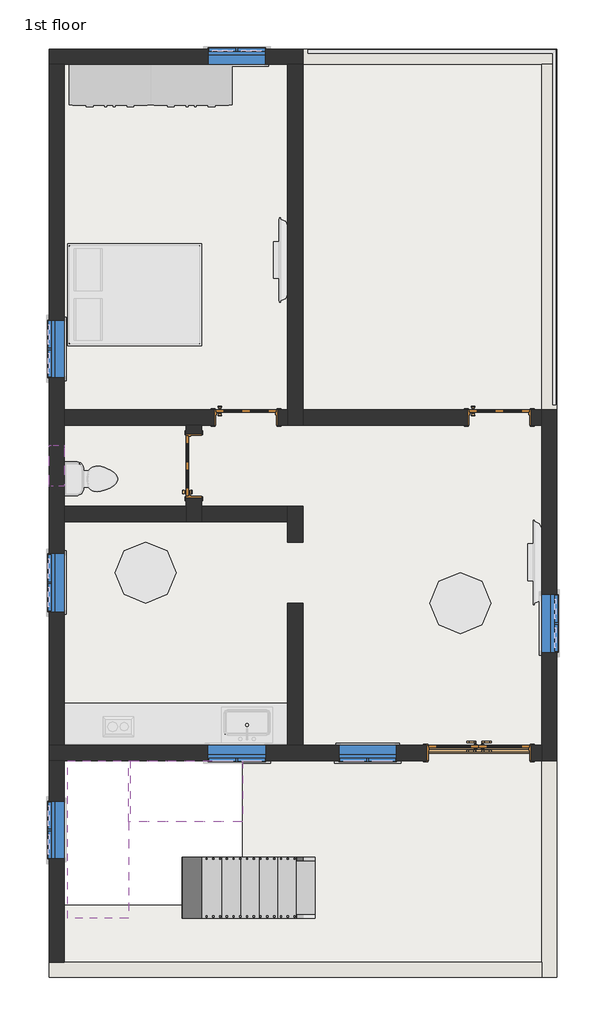
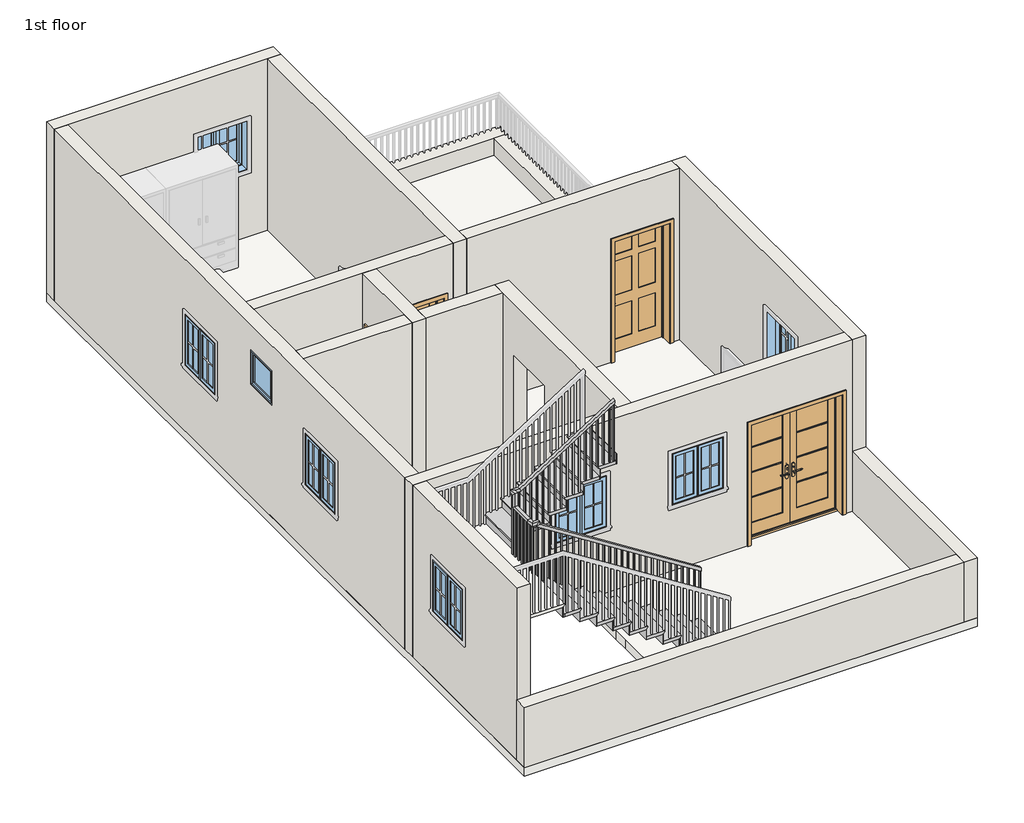
# One storey, part 1 of 3: 16 walls, 8 windows, 4 doors, 2 slabs, 2 stair flights, 1 railing.
"""IFC4 building model written with IfcOpenShell, lengths in millimetres."""

from ifc_helpers import new_model, si_unit, frame, origin, place, context, project, spatial, polyline, outline, extrude, faceted_brep, transform, mapped, element, save
from components import door_7ffae4ec, door_d86b6c54, non_monolithic_landing_094f5741, stair_flight_440f75bd, stair_flight_2f9793b1, window_80340324, window_339605e1

model = new_model("IFC4")

# Units and contexts
model_context = context("Model", 3, world=origin())
ifc_project = project(units=[si_unit("LENGTHUNIT", "METRE", prefix="MILLI")], contexts=[model_context])

# Site, building, storey
site = spatial("IfcSite", under=ifc_project)
building = spatial("IfcBuilding", under=site)
storey = spatial("IfcBuildingStorey", under=building, Name="1st floor", Elevation=3810.0)

# Doors
placement = place(None, origin())
door_shape = door_7ffae4ec(model_context)
element("IfcDoor", 1, ObjectType="Door-Exterior-Double-Full Glass-Wood_Clad : 60\" x 84\"", at=placement, inside=storey, context=model_context, shape_type="MappedRepresentation", body=[
    mapped(door_shape, transform((25464.9136801, 6646.2502787, 3810.0), x_axis=(1.0, 0.0, 0.0), y_axis=(0.0, 1.0, 0.0), z_axis=(0.0, 0.0, 1.0))),
])
door_2_shape = door_d86b6c54(model_context)
element("IfcDoor", 2, ObjectType="Door-Interior-Single-6_Panel-Wood : 36\" x 84\"", at=placement, inside=storey, context=model_context, shape_type="MappedRepresentation", body=[
    mapped(door_2_shape, transform((25769.7136801, 11675.4502787, 3810.0), x_axis=(1.0, 0.0, 0.0), y_axis=(0.0, 1.0, 0.0), z_axis=(0.0, 0.0, 1.0))),
])
element("IfcDoor", 3, ObjectType="Door-Interior-Single-6_Panel-Wood : 36\" x 84\"", at=placement, inside=storey, context=model_context, shape_type="MappedRepresentation", body=[
    mapped(door_2_shape, transform((21969.5484036, 11675.4502787, 3810.0), x_axis=(1.0, 0.0, 0.0), y_axis=(0.0, 1.0, 0.0), z_axis=(0.0, 0.0, 1.0))),
])
element("IfcDoor", 4, ObjectType="Door-Interior-Single-6_Panel-Wood : 36\" x 84\"", at=placement, inside=storey, context=model_context, shape_type="MappedRepresentation", body=[
    mapped(door_2_shape, transform((21181.8386801, 10948.3752787, 3810.0), x_axis=(0.0, 1.0, 0.0), y_axis=(-1.0, 0.0, 0.0), z_axis=(0.0, 0.0, 1.0))),
])

# Railing
element("IfcRailing", 5, ObjectType="Handrail - Rectangular", at=placement, inside=storey, context=model_context, shape_type="SolidModel", body=[
    faceted_brep([(23001.1136801, 5030.1752787, 4902.2), (23001.1136801, 5030.1752787, 4841.986276), (23001.1136801, 5080.9752787, 4841.986276), (23001.1136801, 5080.9752787, 4902.2), (20283.3136801, 5030.1752787, 6631.7090909), (20232.5136801, 5030.1752787, 6603.8226396), (20232.5136801, 5080.9752787, 6603.8226396), (20283.3136801, 5080.9752787, 6631.7090909), (20283.3136801, 5030.1752787, 6680.2), (20232.5136801, 5030.1752787, 6629.4), (20232.5136801, 5080.9752787, 6629.4), (20283.3136801, 5080.9752787, 6680.2), (20156.3136801, 5030.1752787, 6680.2), (20156.3136801, 5030.1752787, 6629.4), (20207.1136801, 5080.9752787, 6629.4), (20207.1136801, 5080.9752787, 6680.2), (20156.3136801, 5157.1752787, 6680.2), (20156.3136801, 5157.1752787, 6629.4), (20207.1136801, 5157.1752787, 6629.4), (20207.1136801, 5157.1752787, 6680.2), (20156.3136801, 5538.1752787, 6680.2), (20156.3136801, 5588.9752787, 6629.4), (20207.1136801, 5588.9752787, 6629.4), (20207.1136801, 5538.1752787, 6680.2), (20156.3136801, 5538.1752787, 6906.4909091), (20156.3136801, 5588.9752787, 6855.6909091), (20207.1136801, 5588.9752787, 6855.6909091), (20207.1136801, 5538.1752787, 6906.4909091), (20156.3136801, 5665.1752787, 6906.4909091), (20156.3136801, 5665.1752787, 6855.6909091), (20207.1136801, 5614.3752787, 6855.6909091), (20207.1136801, 5614.3752787, 6906.4909091), (20283.3136801, 5665.1752787, 6906.4909091), (20298.106675, 5665.1752787, 6855.6909091), (20298.106675, 5614.3752787, 6855.6909091), (20283.3136801, 5614.3752787, 6906.4909091), (21883.5136801, 5665.1752787, 7924.8), (21883.5136801, 5614.3752787, 7924.8), (21883.5136801, 5614.3752787, 7864.586276), (21883.5136801, 5665.1752787, 7864.586276)], [[[0, 1, 2, 3]], [[1, 0, 4, 5]], [[2, 1, 5, 6]], [[3, 2, 6, 7]], [[0, 3, 7, 4]], [[5, 4, 8, 9]], [[6, 5, 9, 10]], [[7, 6, 10, 11]], [[4, 7, 11, 8]], [[9, 8, 12, 13]], [[10, 9, 13, 14]], [[11, 10, 14, 15]], [[8, 11, 15, 12]], [[13, 12, 16, 17]], [[14, 13, 17, 18]], [[15, 14, 18, 19]], [[12, 15, 19, 16]], [[17, 16, 20, 21]], [[18, 17, 21, 22]], [[19, 18, 22, 23]], [[16, 19, 23, 20]], [[21, 20, 24, 25]], [[22, 21, 25, 26]], [[23, 22, 26, 27]], [[20, 23, 27, 24]], [[25, 24, 28, 29]], [[26, 25, 29, 30]], [[27, 26, 30, 31]], [[24, 27, 31, 28]], [[29, 28, 32, 33]], [[30, 29, 33, 34]], [[31, 30, 34, 35]], [[28, 31, 35, 32]], [[36, 37, 38, 39]], [[33, 32, 36, 39]], [[34, 33, 39, 38]], [[35, 34, 38, 37]], [[32, 35, 37, 36]]]),
    extrude(outline(polyline([(7822.1567305, 21816.8386801), (7810.0340032, 21797.7886801), (6832.6, 21797.7886801), (6832.6, 21816.8386801), (7822.1567305, 21816.8386801)])), frame((0.0, 5630.2502787, 0.0), z_axis=(0.0, 1.0, 0.0), x_axis=(0.0, 0.0, 1.0)), (0.0, 0.0, 1.0), 19.05),
    extrude(outline(polyline([(7757.5021851, 21715.2386801), (7745.3794578, 21696.1886801), (6832.6, 21696.1886801), (6832.6, 21715.2386801), (7757.5021851, 21715.2386801)])), frame((0.0, 5630.2502787, 0.0), z_axis=(0.0, 1.0, 0.0), x_axis=(0.0, 0.0, 1.0)), (0.0, 0.0, 1.0), 19.05),
    extrude(outline(polyline([(7692.8476396, 21613.6386801), (7680.7249123, 21594.5886801), (6832.6, 21594.5886801), (6832.6, 21613.6386801), (7692.8476396, 21613.6386801)])), frame((0.0, 5630.2502787, 0.0), z_axis=(0.0, 1.0, 0.0), x_axis=(0.0, 0.0, 1.0)), (0.0, 0.0, 1.0), 19.05),
    extrude(outline(polyline([(7628.1930941, 21512.0386801), (7616.0703669, 21492.9886801), (6654.8, 21492.9886801), (6654.8, 21512.0386801), (7628.1930941, 21512.0386801)])), frame((0.0, 5630.2502787, 0.0), z_axis=(0.0, 1.0, 0.0), x_axis=(0.0, 0.0, 1.0)), (0.0, 0.0, 1.0), 19.05),
    extrude(outline(polyline([(7563.5385487, 21410.4386801), (7551.4158214, 21391.3886801), (6654.8, 21391.3886801), (6654.8, 21410.4386801), (7563.5385487, 21410.4386801)])), frame((0.0, 5630.2502787, 0.0), z_axis=(0.0, 1.0, 0.0), x_axis=(0.0, 0.0, 1.0)), (0.0, 0.0, 1.0), 19.05),
    extrude(outline(polyline([(7498.8840032, 21308.8386801), (7486.761276, 21289.7886801), (6477.0, 21289.7886801), (6477.0, 21308.8386801), (7498.8840032, 21308.8386801)])), frame((0.0, 5630.2502787, 0.0), z_axis=(0.0, 1.0, 0.0), x_axis=(0.0, 0.0, 1.0)), (0.0, 0.0, 1.0), 19.05),
    extrude(outline(polyline([(7434.2294578, 21207.2386801), (7422.1067305, 21188.1886801), (6477.0, 21188.1886801), (6477.0, 21207.2386801), (7434.2294578, 21207.2386801)])), frame((0.0, 5630.2502787, 0.0), z_axis=(0.0, 1.0, 0.0), x_axis=(0.0, 0.0, 1.0)), (0.0, 0.0, 1.0), 19.05),
    extrude(outline(polyline([(7369.5749123, 21105.6386801), (7357.4521851, 21086.5886801), (6477.0, 21086.5886801), (6477.0, 21105.6386801), (7369.5749123, 21105.6386801)])), frame((0.0, 5630.2502787, 0.0), z_axis=(0.0, 1.0, 0.0), x_axis=(0.0, 0.0, 1.0)), (0.0, 0.0, 1.0), 19.05),
    extrude(outline(polyline([(7304.9203669, 21004.0386801), (7292.7976396, 20984.9886801), (6299.2, 20984.9886801), (6299.2, 21004.0386801), (7304.9203669, 21004.0386801)])), frame((0.0, 5630.2502787, 0.0), z_axis=(0.0, 1.0, 0.0), x_axis=(0.0, 0.0, 1.0)), (0.0, 0.0, 1.0), 19.05),
    extrude(outline(polyline([(7240.2658214, 20902.4386801), (7228.1430941, 20883.3886801), (6299.2, 20883.3886801), (6299.2, 20902.4386801), (7240.2658214, 20902.4386801)])), frame((0.0, 5630.2502787, 0.0), z_axis=(0.0, 1.0, 0.0), x_axis=(0.0, 0.0, 1.0)), (0.0, 0.0, 1.0), 19.05),
    extrude(outline(polyline([(7175.611276, 20800.8386801), (7163.4885487, 20781.7886801), (6299.2, 20781.7886801), (6299.2, 20800.8386801), (7175.611276, 20800.8386801)])), frame((0.0, 5630.2502787, 0.0), z_axis=(0.0, 1.0, 0.0), x_axis=(0.0, 0.0, 1.0)), (0.0, 0.0, 1.0), 19.05),
    extrude(outline(polyline([(7110.9567305, 20699.2386801), (7098.8340032, 20680.1886801), (6121.4, 20680.1886801), (6121.4, 20699.2386801), (7110.9567305, 20699.2386801)])), frame((0.0, 5630.2502787, 0.0), z_axis=(0.0, 1.0, 0.0), x_axis=(0.0, 0.0, 1.0)), (0.0, 0.0, 1.0), 19.05),
    extrude(outline(polyline([(7046.3021851, 20597.6386801), (7034.1794578, 20578.5886801), (6121.4, 20578.5886801), (6121.4, 20597.6386801), (7046.3021851, 20597.6386801)])), frame((0.0, 5630.2502787, 0.0), z_axis=(0.0, 1.0, 0.0), x_axis=(0.0, 0.0, 1.0)), (0.0, 0.0, 1.0), 19.05),
    extrude(outline(polyline([(6981.6476396, 20496.0386801), (6969.5249123, 20476.9886801), (6121.4, 20476.9886801), (6121.4, 20496.0386801), (6981.6476396, 20496.0386801)])), frame((0.0, 5630.2502787, 0.0), z_axis=(0.0, 1.0, 0.0), x_axis=(0.0, 0.0, 1.0)), (0.0, 0.0, 1.0), 19.05),
    extrude(outline(polyline([(6916.9930941, 20394.4386801), (6904.8703669, 20375.3886801), (5943.6, 20375.3886801), (5943.6, 20394.4386801), (6916.9930941, 20394.4386801)])), frame((0.0, 5630.2502787, 0.0), z_axis=(0.0, 1.0, 0.0), x_axis=(0.0, 0.0, 1.0)), (0.0, 0.0, 1.0), 19.05),
    extrude(outline(polyline([(6852.3385487, 20292.8386801), (6840.2158214, 20273.7886801), (5943.6, 20273.7886801), (5943.6, 20292.8386801), (6852.3385487, 20292.8386801)])), frame((0.0, 5630.2502787, 0.0), z_axis=(0.0, 1.0, 0.0), x_axis=(0.0, 0.0, 1.0)), (0.0, 0.0, 1.0), 19.05),
    extrude(outline(polyline([(20191.2386801, 5554.0502787), (20172.1886801, 5554.0502787), (20172.1886801, 5573.1002787), (20191.2386801, 5573.1002787), (20191.2386801, 5554.0502787)])), frame((0.0, 0.0, 5765.8), z_axis=(0.0, 0.0, 1.0), x_axis=(1.0, 0.0, 0.0)), (0.0, 0.0, 1.0), 1089.8909091),
    extrude(outline(polyline([(20191.2386801, 5452.4502787), (20172.1886801, 5452.4502787), (20172.1886801, 5471.5002787), (20191.2386801, 5471.5002787), (20191.2386801, 5452.4502787)])), frame((0.0, 0.0, 5765.8), z_axis=(0.0, 0.0, 1.0), x_axis=(1.0, 0.0, 0.0)), (0.0, 0.0, 1.0), 863.6),
    extrude(outline(polyline([(20191.2386801, 5350.8502787), (20172.1886801, 5350.8502787), (20172.1886801, 5369.9002787), (20191.2386801, 5369.9002787), (20191.2386801, 5350.8502787)])), frame((0.0, 0.0, 5765.8), z_axis=(0.0, 0.0, 1.0), x_axis=(1.0, 0.0, 0.0)), (0.0, 0.0, 1.0), 863.6),
    extrude(outline(polyline([(20191.2386801, 5249.2502787), (20172.1886801, 5249.2502787), (20172.1886801, 5268.3002787), (20191.2386801, 5268.3002787), (20191.2386801, 5249.2502787)])), frame((0.0, 0.0, 5765.8), z_axis=(0.0, 0.0, 1.0), x_axis=(1.0, 0.0, 0.0)), (0.0, 0.0, 1.0), 863.6),
    extrude(outline(polyline([(20191.2386801, 5147.6502787), (20172.1886801, 5147.6502787), (20172.1886801, 5166.7002787), (20191.2386801, 5166.7002787), (20191.2386801, 5147.6502787)])), frame((0.0, 0.0, 5765.8), z_axis=(0.0, 0.0, 1.0), x_axis=(1.0, 0.0, 0.0)), (0.0, 0.0, 1.0), 863.6),
    extrude(outline(polyline([(20267.4386801, 5065.1002787), (20267.4386801, 5046.0502787), (20248.3886801, 5046.0502787), (20248.3886801, 5065.1002787), (20267.4386801, 5065.1002787)])), frame((0.0, 0.0, 5588.0), z_axis=(0.0, 0.0, 1.0), x_axis=(1.0, 0.0, 0.0)), (0.0, 0.0, 1.0), 1041.4),
    extrude(outline(polyline([(6516.9430941, 20369.0386801), (6529.0658214, 20349.9886801), (5588.0, 20349.9886801), (5588.0, 20369.0386801), (6516.9430941, 20369.0386801)])), frame((0.0, 5046.0502787, 0.0), z_axis=(0.0, 1.0, 0.0), x_axis=(0.0, 0.0, 1.0)), (0.0, 0.0, 1.0), 19.05),
    extrude(outline(polyline([(6452.2885487, 20470.6386801), (6464.411276, 20451.5886801), (5588.0, 20451.5886801), (5588.0, 20470.6386801), (6452.2885487, 20470.6386801)])), frame((0.0, 5046.0502787, 0.0), z_axis=(0.0, 1.0, 0.0), x_axis=(0.0, 0.0, 1.0)), (0.0, 0.0, 1.0), 19.05),
    extrude(outline(polyline([(6387.6340032, 20572.2386801), (6399.7567305, 20553.1886801), (5410.2, 20553.1886801), (5410.2, 20572.2386801), (6387.6340032, 20572.2386801)])), frame((0.0, 5046.0502787, 0.0), z_axis=(0.0, 1.0, 0.0), x_axis=(0.0, 0.0, 1.0)), (0.0, 0.0, 1.0), 19.05),
    extrude(outline(polyline([(6322.9794578, 20673.8386801), (6335.1021851, 20654.7886801), (5410.2, 20654.7886801), (5410.2, 20673.8386801), (6322.9794578, 20673.8386801)])), frame((0.0, 5046.0502787, 0.0), z_axis=(0.0, 1.0, 0.0), x_axis=(0.0, 0.0, 1.0)), (0.0, 0.0, 1.0), 19.05),
    extrude(outline(polyline([(6258.3249123, 20775.4386801), (6270.4476396, 20756.3886801), (5410.2, 20756.3886801), (5410.2, 20775.4386801), (6258.3249123, 20775.4386801)])), frame((0.0, 5046.0502787, 0.0), z_axis=(0.0, 1.0, 0.0), x_axis=(0.0, 0.0, 1.0)), (0.0, 0.0, 1.0), 19.05),
    extrude(outline(polyline([(6193.6703669, 20877.0386801), (6205.7930941, 20857.9886801), (5232.4, 20857.9886801), (5232.4, 20877.0386801), (6193.6703669, 20877.0386801)])), frame((0.0, 5046.0502787, 0.0), z_axis=(0.0, 1.0, 0.0), x_axis=(0.0, 0.0, 1.0)), (0.0, 0.0, 1.0), 19.05),
    extrude(outline(polyline([(6129.0158214, 20978.6386801), (6141.1385487, 20959.5886801), (5232.4, 20959.5886801), (5232.4, 20978.6386801), (6129.0158214, 20978.6386801)])), frame((0.0, 5046.0502787, 0.0), z_axis=(0.0, 1.0, 0.0), x_axis=(0.0, 0.0, 1.0)), (0.0, 0.0, 1.0), 19.05),
    extrude(outline(polyline([(6064.361276, 21080.2386801), (6076.4840032, 21061.1886801), (5054.6, 21061.1886801), (5054.6, 21080.2386801), (6064.361276, 21080.2386801)])), frame((0.0, 5046.0502787, 0.0), z_axis=(0.0, 1.0, 0.0), x_axis=(0.0, 0.0, 1.0)), (0.0, 0.0, 1.0), 19.05),
    extrude(outline(polyline([(5999.7067305, 21181.8386801), (6011.8294578, 21162.7886801), (5054.6, 21162.7886801), (5054.6, 21181.8386801), (5999.7067305, 21181.8386801)])), frame((0.0, 5046.0502787, 0.0), z_axis=(0.0, 1.0, 0.0), x_axis=(0.0, 0.0, 1.0)), (0.0, 0.0, 1.0), 19.05),
    extrude(outline(polyline([(5935.0521851, 21283.4386801), (5947.1749123, 21264.3886801), (5054.6, 21264.3886801), (5054.6, 21283.4386801), (5935.0521851, 21283.4386801)])), frame((0.0, 5046.0502787, 0.0), z_axis=(0.0, 1.0, 0.0), x_axis=(0.0, 0.0, 1.0)), (0.0, 0.0, 1.0), 19.05),
    extrude(outline(polyline([(5870.3976396, 21385.0386801), (5882.5203669, 21365.9886801), (4876.8, 21365.9886801), (4876.8, 21385.0386801), (5870.3976396, 21385.0386801)])), frame((0.0, 5046.0502787, 0.0), z_axis=(0.0, 1.0, 0.0), x_axis=(0.0, 0.0, 1.0)), (0.0, 0.0, 1.0), 19.05),
    extrude(outline(polyline([(5805.7430941, 21486.6386801), (5817.8658214, 21467.5886801), (4876.8, 21467.5886801), (4876.8, 21486.6386801), (5805.7430941, 21486.6386801)])), frame((0.0, 5046.0502787, 0.0), z_axis=(0.0, 1.0, 0.0), x_axis=(0.0, 0.0, 1.0)), (0.0, 0.0, 1.0), 19.05),
    extrude(outline(polyline([(5741.0885487, 21588.2386801), (5753.211276, 21569.1886801), (4876.8, 21569.1886801), (4876.8, 21588.2386801), (5741.0885487, 21588.2386801)])), frame((0.0, 5046.0502787, 0.0), z_axis=(0.0, 1.0, 0.0), x_axis=(0.0, 0.0, 1.0)), (0.0, 0.0, 1.0), 19.05),
    extrude(outline(polyline([(5676.4340032, 21689.8386801), (5688.5567305, 21670.7886801), (4699.0, 21670.7886801), (4699.0, 21689.8386801), (5676.4340032, 21689.8386801)])), frame((0.0, 5046.0502787, 0.0), z_axis=(0.0, 1.0, 0.0), x_axis=(0.0, 0.0, 1.0)), (0.0, 0.0, 1.0), 19.05),
    extrude(outline(polyline([(5611.7794578, 21791.4386801), (5623.9021851, 21772.3886801), (4699.0, 21772.3886801), (4699.0, 21791.4386801), (5611.7794578, 21791.4386801)])), frame((0.0, 5046.0502787, 0.0), z_axis=(0.0, 1.0, 0.0), x_axis=(0.0, 0.0, 1.0)), (0.0, 0.0, 1.0), 19.05),
    extrude(outline(polyline([(5547.1249123, 21893.0386801), (5559.2476396, 21873.9886801), (4699.0, 21873.9886801), (4699.0, 21893.0386801), (5547.1249123, 21893.0386801)])), frame((0.0, 5046.0502787, 0.0), z_axis=(0.0, 1.0, 0.0), x_axis=(0.0, 0.0, 1.0)), (0.0, 0.0, 1.0), 19.05),
    extrude(outline(polyline([(5482.4703669, 21994.6386801), (5494.5930941, 21975.5886801), (4521.2, 21975.5886801), (4521.2, 21994.6386801), (5482.4703669, 21994.6386801)])), frame((0.0, 5046.0502787, 0.0), z_axis=(0.0, 1.0, 0.0), x_axis=(0.0, 0.0, 1.0)), (0.0, 0.0, 1.0), 19.05),
    extrude(outline(polyline([(5417.8158214, 22096.2386801), (5429.9385487, 22077.1886801), (4521.2, 22077.1886801), (4521.2, 22096.2386801), (5417.8158214, 22096.2386801)])), frame((0.0, 5046.0502787, 0.0), z_axis=(0.0, 1.0, 0.0), x_axis=(0.0, 0.0, 1.0)), (0.0, 0.0, 1.0), 19.05),
    extrude(outline(polyline([(5353.161276, 22197.8386801), (5365.2840032, 22178.7886801), (4343.4, 22178.7886801), (4343.4, 22197.8386801), (5353.161276, 22197.8386801)])), frame((0.0, 5046.0502787, 0.0), z_axis=(0.0, 1.0, 0.0), x_axis=(0.0, 0.0, 1.0)), (0.0, 0.0, 1.0), 19.05),
    extrude(outline(polyline([(5288.5067305, 22299.4386801), (5300.6294578, 22280.3886801), (4343.4, 22280.3886801), (4343.4, 22299.4386801), (5288.5067305, 22299.4386801)])), frame((0.0, 5046.0502787, 0.0), z_axis=(0.0, 1.0, 0.0), x_axis=(0.0, 0.0, 1.0)), (0.0, 0.0, 1.0), 19.05),
    extrude(outline(polyline([(5223.8521851, 22401.0386801), (5235.9749123, 22381.9886801), (4343.4, 22381.9886801), (4343.4, 22401.0386801), (5223.8521851, 22401.0386801)])), frame((0.0, 5046.0502787, 0.0), z_axis=(0.0, 1.0, 0.0), x_axis=(0.0, 0.0, 1.0)), (0.0, 0.0, 1.0), 19.05),
    extrude(outline(polyline([(5159.1976396, 22502.6386801), (5171.3203669, 22483.5886801), (4165.6, 22483.5886801), (4165.6, 22502.6386801), (5159.1976396, 22502.6386801)])), frame((0.0, 5046.0502787, 0.0), z_axis=(0.0, 1.0, 0.0), x_axis=(0.0, 0.0, 1.0)), (0.0, 0.0, 1.0), 19.05),
    extrude(outline(polyline([(5094.5430941, 22604.2386801), (5106.6658214, 22585.1886801), (4165.6, 22585.1886801), (4165.6, 22604.2386801), (5094.5430941, 22604.2386801)])), frame((0.0, 5046.0502787, 0.0), z_axis=(0.0, 1.0, 0.0), x_axis=(0.0, 0.0, 1.0)), (0.0, 0.0, 1.0), 19.05),
    extrude(outline(polyline([(5029.8885487, 22705.8386801), (5042.011276, 22686.7886801), (4165.6, 22686.7886801), (4165.6, 22705.8386801), (5029.8885487, 22705.8386801)])), frame((0.0, 5046.0502787, 0.0), z_axis=(0.0, 1.0, 0.0), x_axis=(0.0, 0.0, 1.0)), (0.0, 0.0, 1.0), 19.05),
    extrude(outline(polyline([(4965.2340032, 22807.4386801), (4977.3567305, 22788.3886801), (3987.8, 22788.3886801), (3987.8, 22807.4386801), (4965.2340032, 22807.4386801)])), frame((0.0, 5046.0502787, 0.0), z_axis=(0.0, 1.0, 0.0), x_axis=(0.0, 0.0, 1.0)), (0.0, 0.0, 1.0), 19.05),
    extrude(outline(polyline([(4900.5794578, 22909.0386801), (4912.7021851, 22889.9886801), (3987.8, 22889.9886801), (3987.8, 22909.0386801), (4900.5794578, 22909.0386801)])), frame((0.0, 5046.0502787, 0.0), z_axis=(0.0, 1.0, 0.0), x_axis=(0.0, 0.0, 1.0)), (0.0, 0.0, 1.0), 19.05),
    extrude(outline(polyline([(20191.2386801, 5630.2502787), (20172.1886801, 5630.2502787), (20172.1886801, 5649.3002787), (20191.2386801, 5649.3002787), (20191.2386801, 5630.2502787)])), frame((0.0, 0.0, 5765.8), z_axis=(0.0, 0.0, 1.0), x_axis=(1.0, 0.0, 0.0)), (0.0, 0.0, 1.0), 1089.8909091),
    extrude(outline(polyline([(20191.2386801, 5065.1002787), (20191.2386801, 5046.0502787), (20172.1886801, 5046.0502787), (20172.1886801, 5065.1002787), (20191.2386801, 5065.1002787)])), frame((0.0, 0.0, 5765.8), z_axis=(0.0, 0.0, 1.0), x_axis=(1.0, 0.0, 0.0)), (0.0, 0.0, 1.0), 863.6),
    extrude(outline(polyline([(7864.586276, 21883.5136801), (7852.4635487, 21864.4636801), (6832.6, 21864.4636801), (6832.6, 21883.5136801), (7864.586276, 21883.5136801)])), frame((0.0, 5630.2502787, 0.0), z_axis=(0.0, 1.0, 0.0), x_axis=(0.0, 0.0, 1.0)), (0.0, 0.0, 1.0), 19.05),
    extrude(outline(polyline([(4841.986276, 23001.1136801), (4854.1090032, 22982.0636801), (3987.8, 22982.0636801), (3987.8, 23001.1136801), (4841.986276, 23001.1136801)])), frame((0.0, 5046.0502787, 0.0), z_axis=(0.0, 1.0, 0.0), x_axis=(0.0, 0.0, 1.0)), (0.0, 0.0, 1.0), 19.05),
])

# Slabs
element("IfcSlab", 6, at=placement, inside=storey, context=model_context, shape_type="SweptSolid", body=[
    extrude(outline(polyline([(26633.3136801, 17196.7752787), (26633.3136801, 3277.5752787), (19013.3136801, 3277.5752787), (19013.3136801, 17196.7752787), (26633.3136801, 17196.7752787)]), holes=[polyline([(19241.9136801, 6724.5096261), (19241.9136801, 4369.7752787), (21908.9136801, 4369.7752787), (21908.9136801, 5360.3752787), (21908.9136801, 5614.3752787), (21908.9136801, 6724.5096261), (19241.9136801, 6724.5096261)])]), frame((0.0, 0.0, 3657.6), z_axis=(0.0, 0.0, 1.0), x_axis=(1.0, 0.0, 0.0)), (0.0, 0.0, 1.0), 152.4),
])
non_monolithic_landing_shape = non_monolithic_landing_094f5741(model_context)
element("IfcSlab", 7, ObjectType="Non-Monolithic Landing", at=placement, inside=storey, context=model_context, shape_type="MappedRepresentation", body=[
    mapped(non_monolithic_landing_shape, transform((0.0, 0.0, 0.0), x_axis=(1.0, 0.0, 0.0), y_axis=(0.0, 1.0, 0.0), z_axis=(0.0, 0.0, 1.0))),
])

# Stair flights
stair_flight_shape = stair_flight_440f75bd(model_context)
element("IfcStairFlight", 8, ObjectType="2\" Tread 1\" Nosing 1/4\" Riser", at=placement, inside=storey, context=model_context, shape_type="MappedRepresentation", body=[
    mapped(stair_flight_shape, transform((0.0, 0.0, 0.0), x_axis=(1.0, 0.0, 0.0), y_axis=(0.0, 1.0, 0.0), z_axis=(0.0, 0.0, 1.0))),
])
stair_flight_2_shape = stair_flight_2f9793b1(model_context)
element("IfcStairFlight", 9, ObjectType="2\" Tread 1\" Nosing 1/4\" Riser", at=placement, inside=storey, context=model_context, shape_type="MappedRepresentation", body=[
    mapped(stair_flight_2_shape, transform((0.0, 0.0, 0.0), x_axis=(1.0, 0.0, 0.0), y_axis=(0.0, 1.0, 0.0), z_axis=(0.0, 0.0, 1.0))),
])

# Walls
element("IfcWall", 10, at=placement, inside=storey, context=model_context, shape_type="Brep", body=[
    faceted_brep([(19013.3136801, 16968.1752787, 3810.0), (19241.9136801, 16968.1752787, 3810.0), (22594.7136801, 16968.1752787, 3810.0), (22709.0136801, 16968.1752787, 3810.0), (22709.0136801, 16968.1752787, 4114.8), (22823.3136801, 16968.1752787, 4114.8), (22823.3136801, 16968.1752787, 6858.0), (22594.7136801, 16968.1752787, 6858.0), (19241.9136801, 16968.1752787, 6858.0), (19013.3136801, 16968.1752787, 6858.0), (22264.5136801, 16968.1752787, 5908.675), (22264.5136801, 16968.1752787, 4994.275), (21400.9136801, 16968.1752787, 4994.275), (21400.9136801, 16968.1752787, 5908.675), (19013.3136801, 17196.7752787, 3810.0), (19013.3136801, 17196.7752787, 6858.0), (22823.3136801, 17196.7752787, 6858.0), (22823.3136801, 17196.7752787, 4114.8), (22709.0136801, 17196.7752787, 4114.8), (22709.0136801, 17196.7752787, 3810.0), (22264.5136801, 17196.7752787, 5908.675), (21400.9136801, 17196.7752787, 5908.675), (21400.9136801, 17196.7752787, 4994.275), (22264.5136801, 17196.7752787, 4994.275)], [[[0, 1, 2, 3, 4, 5, 6, 7, 8, 9], [10, 11, 12, 13]], [[14, 15, 16, 17, 18, 19], [20, 21, 22, 23]], [[3, 2, 1, 0, 14, 19]], [[0, 9, 15, 14]], [[11, 10, 20, 23]], [[12, 11, 23, 22]], [[13, 12, 22, 21]], [[10, 13, 21, 20]], [[4, 3, 19, 18]], [[17, 5, 4, 18]], [[6, 5, 17, 16]], [[9, 8, 7, 6, 16, 15]]]),
])
element("IfcWall", 11, at=placement, inside=storey, context=model_context, shape_type="Brep", body=[
    faceted_brep([(26404.7136801, 16968.1752787, 3810.0), (26404.7136801, 11786.5752787, 3810.0), (26404.7136801, 11672.2752787, 3810.0), (26404.7136801, 11672.2752787, 4114.8), (26404.7136801, 11786.5752787, 4114.8), (26404.7136801, 16968.1752787, 4114.8), (26633.3136801, 16968.1752787, 3810.0), (26633.3136801, 16968.1752787, 4114.8), (26633.3136801, 11786.5752787, 4114.8), (26633.3136801, 11672.2752787, 4114.8), (26633.3136801, 11672.2752787, 3810.0)], [[[0, 1, 2, 3, 4, 5]], [[6, 7, 8, 9, 10]], [[2, 1, 0, 6, 10]], [[3, 2, 10, 9]], [[5, 4, 3, 9, 8, 7]], [[0, 5, 7, 6]]]),
])
element("IfcWall", 12, at=placement, inside=storey, context=model_context, shape_type="Brep", body=[
    faceted_brep([(26404.7136801, 3506.1752787, 3810.0), (19241.9136801, 3506.1752787, 3810.0), (19013.3136801, 3506.1752787, 3810.0), (19013.3136801, 3506.1752787, 4876.8), (26404.7136801, 3506.1752787, 4876.8), (26404.7136801, 3277.5752787, 3810.0), (26404.7136801, 3277.5752787, 4876.8), (19013.3136801, 3277.5752787, 4876.8), (19013.3136801, 3277.5752787, 3810.0)], [[[0, 1, 2, 3, 4]], [[5, 6, 7, 8]], [[2, 1, 0, 5, 8]], [[4, 3, 7, 6]], [[0, 4, 6, 5]], [[3, 2, 8, 7]]]),
])
element("IfcWall", 13, at=placement, inside=storey, context=model_context, shape_type="Brep", body=[
    faceted_brep([(19241.9136801, 3506.1752787, 3810.0), (19241.9136801, 6528.7752787, 3810.0), (19241.9136801, 6528.7752787, 6858.0), (19241.9136801, 4182.4502787, 6858.0), (19241.9136801, 3506.1752787, 6858.0), (19241.9136801, 5919.1752787, 5908.675), (19241.9136801, 5919.1752787, 4994.275), (19241.9136801, 5055.5752787, 4994.275), (19241.9136801, 5055.5752787, 5908.675), (19013.3136801, 6528.7752787, 3810.0), (19013.3136801, 3506.1752787, 3810.0), (19013.3136801, 3506.1752787, 4876.8), (19013.3136801, 3506.1752787, 6858.0), (19013.3136801, 6528.7752787, 6858.0), (19013.3136801, 5919.1752787, 4994.275), (19013.3136801, 5919.1752787, 5908.675), (19013.3136801, 5055.5752787, 5908.675), (19013.3136801, 5055.5752787, 4994.275)], [[[0, 1, 2, 3, 4], [5, 6, 7, 8]], [[9, 10, 11, 12, 13], [14, 15, 16, 17]], [[1, 0, 10, 9]], [[0, 4, 12, 11, 10]], [[2, 1, 9, 13]], [[5, 15, 14, 6]], [[6, 14, 17, 7]], [[7, 17, 16, 8]], [[15, 5, 8, 16]], [[13, 12, 4, 3, 2]]]),
])
element("IfcWall", 14, at=placement, inside=storey, context=model_context, shape_type="Brep", body=[
    faceted_brep([(22594.7136801, 16968.1752787, 6858.0), (22594.7136801, 16968.1752787, 3810.0), (22594.7136801, 11786.5752787, 3810.0), (22594.7136801, 11557.9752787, 3810.0), (22594.7136801, 11557.9752787, 6858.0), (22594.7136801, 11786.5752787, 6858.0), (22823.3136801, 16968.1752787, 3810.0), (22823.3136801, 16968.1752787, 4114.8), (22823.3136801, 16968.1752787, 6858.0), (22823.3136801, 11786.5752787, 6858.0), (22823.3136801, 11557.9752787, 6858.0), (22823.3136801, 11557.9752787, 3810.0), (22823.3136801, 11786.5752787, 3810.0), (22709.0136801, 16968.1752787, 3810.0)], [[[0, 1, 2, 3, 4, 5]], [[6, 7, 8, 9, 10, 11, 12]], [[3, 2, 1, 13, 6, 12, 11]], [[4, 3, 11, 10]], [[0, 8, 7, 6, 13, 1]], [[0, 5, 4, 10, 9, 8]]]),
])
element("IfcWall", 15, at=placement, inside=storey, context=model_context, shape_type="Brep", body=[
    faceted_brep([(22594.7136801, 11786.5752787, 6858.0), (22594.7136801, 11786.5752787, 3810.0), (22452.1484036, 11786.5752787, 3810.0), (22452.1484036, 11786.5752787, 5969.0), (21486.9484036, 11786.5752787, 5969.0), (21486.9484036, 11786.5752787, 3810.0), (19241.9136801, 11786.5752787, 3810.0), (19241.9136801, 11786.5752787, 6858.0), (22594.7136801, 11557.9752787, 3810.0), (22594.7136801, 11557.9752787, 6858.0), (21299.3136801, 11557.9752787, 6858.0), (21070.7136801, 11557.9752787, 6858.0), (19241.9136801, 11557.9752787, 6858.0), (19241.9136801, 11557.9752787, 3810.0), (21070.7136801, 11557.9752787, 3810.0), (21299.3136801, 11557.9752787, 3810.0), (21486.9484036, 11557.9752787, 3810.0), (21486.9484036, 11557.9752787, 5969.0), (22452.1484036, 11557.9752787, 5969.0), (22452.1484036, 11557.9752787, 3810.0)], [[[0, 1, 2, 3, 4, 5, 6, 7]], [[8, 9, 10, 11, 12, 13, 14, 15, 16, 17, 18, 19]], [[1, 8, 19, 2]], [[13, 6, 5, 16, 15, 14]], [[1, 0, 9, 8]], [[7, 6, 13, 12]], [[18, 3, 2, 19]], [[3, 18, 17, 4]], [[4, 17, 16, 5]], [[0, 7, 12, 11, 10, 9]]]),
])
element("IfcWall", 16, at=placement, inside=storey, context=model_context, shape_type="Brep", body=[
    faceted_brep([(22823.3136801, 11557.9752787, 6858.0), (22823.3136801, 11557.9752787, 3810.0), (25287.1136801, 11557.9752787, 3810.0), (25287.1136801, 11557.9752787, 5969.0), (26252.3136801, 11557.9752787, 5969.0), (26252.3136801, 11557.9752787, 3810.0), (26404.7136801, 11557.9752787, 3810.0), (26404.7136801, 11557.9752787, 6858.0), (22823.3136801, 11786.5752787, 3810.0), (22823.3136801, 11786.5752787, 6858.0), (26404.7136801, 11786.5752787, 6858.0), (26404.7136801, 11786.5752787, 4114.8), (26404.7136801, 11786.5752787, 3810.0), (26252.3136801, 11786.5752787, 3810.0), (26252.3136801, 11786.5752787, 5969.0), (25287.1136801, 11786.5752787, 5969.0), (25287.1136801, 11786.5752787, 3810.0), (26404.7136801, 11672.2752787, 3810.0)], [[[0, 1, 2, 3, 4, 5, 6, 7]], [[8, 9, 10, 11, 12, 13, 14, 15, 16]], [[1, 8, 16, 2]], [[12, 17, 6, 5, 13]], [[1, 0, 9, 8]], [[4, 14, 13, 5]], [[14, 4, 3, 15]], [[15, 3, 2, 16]], [[6, 17, 12, 11, 10, 7]], [[0, 7, 10, 9]]]),
])
element("IfcWall", 17, at=placement, inside=storey, context=model_context, shape_type="Brep", body=[
    faceted_brep([(21070.7136801, 11557.9752787, 6858.0), (21070.7136801, 11557.9752787, 3810.0), (21070.7136801, 11430.9752787, 3810.0), (21070.7136801, 11430.9752787, 5969.0), (21070.7136801, 10465.7752787, 5969.0), (21070.7136801, 10465.7752787, 3810.0), (21070.7136801, 10338.7752787, 3810.0), (21070.7136801, 10110.1752787, 3810.0), (21070.7136801, 10110.1752787, 6858.0), (21070.7136801, 10338.7752787, 6858.0), (21299.3136801, 11557.9752787, 3810.0), (21299.3136801, 11557.9752787, 6858.0), (21299.3136801, 10338.7752787, 6858.0), (21299.3136801, 10110.1752787, 6858.0), (21299.3136801, 10110.1752787, 3810.0), (21299.3136801, 10338.7752787, 3810.0), (21299.3136801, 10465.7752787, 3810.0), (21299.3136801, 10465.7752787, 5969.0), (21299.3136801, 11430.9752787, 5969.0), (21299.3136801, 11430.9752787, 3810.0)], [[[0, 1, 2, 3, 4, 5, 6, 7, 8, 9]], [[10, 11, 12, 13, 14, 15, 16, 17, 18, 19]], [[1, 10, 19, 2]], [[14, 7, 6, 5, 16, 15]], [[1, 0, 11, 10]], [[8, 7, 14, 13]], [[18, 3, 2, 19]], [[3, 18, 17, 4]], [[4, 17, 16, 5]], [[0, 9, 8, 13, 12, 11]]]),
])
element("IfcWall", 18, at=placement, inside=storey, context=model_context, shape_type="SweptSolid", body=[
    extrude(outline(polyline([(19241.9136801, 10338.7752787), (21070.7136801, 10338.7752787), (21070.7136801, 10110.1752787), (19241.9136801, 10110.1752787), (19241.9136801, 10338.7752787)])), frame((0.0, 0.0, 3810.0), z_axis=(0.0, 0.0, 1.0), x_axis=(1.0, 0.0, 0.0)), (0.0, 0.0, 1.0), 3048.0),
])
element("IfcWall", 19, at=placement, inside=storey, context=model_context, shape_type="Brep", body=[
    faceted_brep([(22594.7136801, 10338.7752787, 6858.0), (22594.7136801, 10338.7752787, 3810.0), (22594.7136801, 10110.1752787, 3810.0), (22594.7136801, 9805.3752787, 3810.0), (22594.7136801, 9805.3752787, 5943.6), (22594.7136801, 8890.9752787, 5943.6), (22594.7136801, 8890.9752787, 3810.0), (22594.7136801, 6757.3752787, 3810.0), (22594.7136801, 6757.3752787, 6858.0), (22594.7136801, 10110.1752787, 6858.0), (22823.3136801, 10338.7752787, 3810.0), (22823.3136801, 10338.7752787, 6858.0), (22823.3136801, 6757.3752787, 6858.0), (22823.3136801, 6757.3752787, 3810.0), (22823.3136801, 8890.9752787, 3810.0), (22823.3136801, 8890.9752787, 5943.6), (22823.3136801, 9805.3752787, 5943.6), (22823.3136801, 9805.3752787, 3810.0)], [[[0, 1, 2, 3, 4, 5, 6, 7, 8, 9]], [[10, 11, 12, 13, 14, 15, 16, 17]], [[1, 10, 17, 3, 2]], [[13, 7, 6, 14]], [[1, 0, 11, 10]], [[8, 7, 13, 12]], [[16, 4, 3, 17]], [[5, 15, 14, 6]], [[4, 16, 15, 5]], [[0, 9, 8, 12, 11]]]),
])
element("IfcWall", 20, at=placement, inside=storey, context=model_context, shape_type="SweptSolid", body=[
    extrude(outline(polyline([(22594.7136801, 10110.1752787), (21299.3136801, 10110.1752787), (21299.3136801, 10338.7752787), (22594.7136801, 10338.7752787), (22594.7136801, 10110.1752787)])), frame((0.0, 0.0, 3810.0), z_axis=(0.0, 0.0, 1.0), x_axis=(1.0, 0.0, 0.0)), (0.0, 0.0, 1.0), 3048.0),
])
element("IfcWall", 21, at=placement, inside=storey, context=model_context, shape_type="Brep", body=[
    faceted_brep([(26404.7136801, 6528.7752787, 3810.0), (26404.7136801, 6528.7752787, 6858.0), (21915.2636801, 6528.7752787, 6858.0), (19241.9136801, 6528.7752787, 6858.0), (19013.3136801, 6528.7752787, 6858.0), (19013.3136801, 6528.7752787, 3810.0), (19241.9136801, 6528.7752787, 3810.0), (24677.5136801, 6528.7752787, 3810.0), (24677.5136801, 6528.7752787, 5969.0), (26252.3136801, 6528.7752787, 5969.0), (26252.3136801, 6528.7752787, 3810.0), (23363.0636801, 6528.7752787, 5908.675), (24226.6636801, 6528.7752787, 5908.675), (24226.6636801, 6528.7752787, 4994.275), (23363.0636801, 6528.7752787, 4994.275), (21400.9136801, 6528.7752787, 5908.675), (22264.5136801, 6528.7752787, 5908.675), (22264.5136801, 6528.7752787, 4994.275), (21400.9136801, 6528.7752787, 4994.275), (19013.3136801, 6757.3752787, 6858.0), (19241.9136801, 6757.3752787, 6858.0), (22594.7136801, 6757.3752787, 6858.0), (22823.3136801, 6757.3752787, 6858.0), (26404.7136801, 6757.3752787, 6858.0), (26404.7136801, 6757.3752787, 3810.0), (26252.3136801, 6757.3752787, 3810.0), (26252.3136801, 6757.3752787, 5969.0), (24677.5136801, 6757.3752787, 5969.0), (24677.5136801, 6757.3752787, 3810.0), (22823.3136801, 6757.3752787, 3810.0), (22594.7136801, 6757.3752787, 3810.0), (19241.9136801, 6757.3752787, 3810.0), (19013.3136801, 6757.3752787, 3810.0), (23363.0636801, 6757.3752787, 5908.675), (23363.0636801, 6757.3752787, 4994.275), (24226.6636801, 6757.3752787, 4994.275), (24226.6636801, 6757.3752787, 5908.675), (21400.9136801, 6757.3752787, 5908.675), (21400.9136801, 6757.3752787, 4994.275), (22264.5136801, 6757.3752787, 4994.275), (22264.5136801, 6757.3752787, 5908.675)], [[[0, 1, 2, 3, 4, 5, 6, 7, 8, 9, 10], [11, 12, 13, 14], [15, 16, 17, 18]], [[19, 20, 21, 22, 23, 24, 25, 26, 27, 28, 29, 30, 31, 32], [33, 34, 35, 36], [37, 38, 39, 40]], [[24, 0, 10, 25]], [[5, 32, 31, 30, 29, 28, 7, 6]], [[0, 24, 23, 1]], [[5, 4, 19, 32]], [[9, 26, 25, 10]], [[26, 9, 8, 27]], [[27, 8, 7, 28]], [[34, 33, 11, 14]], [[35, 34, 14, 13]], [[36, 35, 13, 12]], [[33, 36, 12, 11]], [[38, 37, 15, 18]], [[39, 38, 18, 17]], [[40, 39, 17, 16]], [[37, 40, 16, 15]], [[23, 22, 21, 20, 19, 4, 3, 2, 1]]]),
])
element("IfcWall", 22, at=placement, inside=storey, context=model_context, shape_type="Brep", body=[
    faceted_brep([(26404.7136801, 6528.7752787, 3810.0), (26404.7136801, 3506.1752787, 3810.0), (26404.7136801, 3277.5752787, 3810.0), (26404.7136801, 3277.5752787, 4876.8), (26404.7136801, 3506.1752787, 4876.8), (26404.7136801, 6528.7752787, 4876.8), (26633.3136801, 6528.7752787, 3810.0), (26633.3136801, 6528.7752787, 4876.8), (26633.3136801, 3277.5752787, 4876.8), (26633.3136801, 3277.5752787, 3810.0)], [[[0, 1, 2, 3, 4, 5]], [[6, 7, 8, 9]], [[2, 1, 0, 6, 9]], [[5, 4, 3, 8, 7]], [[3, 2, 9, 8]], [[0, 5, 7, 6]]]),
])
element("IfcWall", 23, at=placement, inside=storey, context=model_context, shape_type="Brep", body=[
    faceted_brep([(19241.9136801, 6757.3752787, 3810.0), (19241.9136801, 10110.1752787, 3810.0), (19241.9136801, 10338.7752787, 3810.0), (19241.9136801, 11557.9752787, 3810.0), (19241.9136801, 11786.5752787, 3810.0), (19241.9136801, 16968.1752787, 3810.0), (19241.9136801, 16968.1752787, 6858.0), (19241.9136801, 11786.5752787, 6858.0), (19241.9136801, 11557.9752787, 6858.0), (19241.9136801, 10338.7752787, 6858.0), (19241.9136801, 10110.1752787, 6858.0), (19241.9136801, 6757.3752787, 6858.0), (19241.9136801, 13132.7752787, 5908.675), (19241.9136801, 13132.7752787, 4994.275), (19241.9136801, 12269.1752787, 4994.275), (19241.9136801, 12269.1752787, 5908.675), (19241.9136801, 9627.5752787, 5908.675), (19241.9136801, 9627.5752787, 4994.275), (19241.9136801, 8763.9752787, 4994.275), (19241.9136801, 8763.9752787, 5908.675), (19241.9136801, 11253.1752787, 6400.8), (19241.9136801, 11253.1752787, 5791.2), (19241.9136801, 10643.5752787, 5791.2), (19241.9136801, 10643.5752787, 6400.8), (19013.3136801, 6757.3752787, 3810.0), (19013.3136801, 6757.3752787, 6858.0), (19013.3136801, 16968.1752787, 6858.0), (19013.3136801, 16968.1752787, 3810.0), (19013.3136801, 13132.7752787, 5908.675), (19013.3136801, 12269.1752787, 5908.675), (19013.3136801, 12269.1752787, 4994.275), (19013.3136801, 13132.7752787, 4994.275), (19013.3136801, 9627.5752787, 5908.675), (19013.3136801, 8763.9752787, 5908.675), (19013.3136801, 8763.9752787, 4994.275), (19013.3136801, 9627.5752787, 4994.275), (19013.3136801, 11253.1752787, 6400.8), (19013.3136801, 10643.5752787, 6400.8), (19013.3136801, 10643.5752787, 5791.2), (19013.3136801, 11253.1752787, 5791.2)], [[[0, 1, 2, 3, 4, 5, 6, 7, 8, 9, 10, 11], [12, 13, 14, 15], [16, 17, 18, 19], [20, 21, 22, 23]], [[24, 25, 26, 27], [28, 29, 30, 31], [32, 33, 34, 35], [36, 37, 38, 39]], [[5, 4, 3, 2, 1, 0, 24, 27]], [[6, 5, 27, 26]], [[0, 11, 25, 24]], [[13, 12, 28, 31]], [[14, 13, 31, 30]], [[15, 14, 30, 29]], [[12, 15, 29, 28]], [[17, 16, 32, 35]], [[18, 17, 35, 34]], [[19, 18, 34, 33]], [[16, 19, 33, 32]], [[21, 20, 36, 39]], [[22, 21, 39, 38]], [[23, 22, 38, 37]], [[20, 23, 37, 36]], [[11, 10, 9, 8, 7, 6, 26, 25]]]),
])
element("IfcWall", 24, at=placement, inside=storey, context=model_context, shape_type="Brep", body=[
    faceted_brep([(22709.0136801, 16968.1752787, 3810.0), (22823.3136801, 16968.1752787, 3810.0), (26404.7136801, 16968.1752787, 3810.0), (26633.3136801, 16968.1752787, 3810.0), (26633.3136801, 16968.1752787, 4114.8), (26404.7136801, 16968.1752787, 4114.8), (22823.3136801, 16968.1752787, 4114.8), (22709.0136801, 16968.1752787, 4114.8), (22709.0136801, 17196.7752787, 3810.0), (22709.0136801, 17196.7752787, 4114.8), (22823.3136801, 17196.7752787, 4114.8), (26633.3136801, 17196.7752787, 4114.8), (26633.3136801, 17196.7752787, 3810.0)], [[[0, 1, 2, 3, 4, 5, 6, 7]], [[8, 9, 10, 11, 12]], [[3, 2, 1, 0, 8, 12]], [[7, 6, 5, 4, 11, 10, 9]], [[0, 7, 9, 8]], [[4, 3, 12, 11]]]),
])
element("IfcWall", 25, at=placement, inside=storey, context=model_context, shape_type="Brep", body=[
    faceted_brep([(26404.7136801, 11672.2752787, 3810.0), (26404.7136801, 11557.9752787, 3810.0), (26404.7136801, 6757.3752787, 3810.0), (26404.7136801, 6528.7752787, 3810.0), (26404.7136801, 6528.7752787, 4876.8), (26404.7136801, 6528.7752787, 6858.0), (26404.7136801, 6757.3752787, 6858.0), (26404.7136801, 11557.9752787, 6858.0), (26404.7136801, 11786.5752787, 6858.0), (26404.7136801, 11786.5752787, 4114.8), (26404.7136801, 11672.2752787, 4114.8), (26404.7136801, 8154.3752787, 5908.675), (26404.7136801, 8154.3752787, 4994.275), (26404.7136801, 9017.9752787, 4994.275), (26404.7136801, 9017.9752787, 5908.675), (26633.3136801, 11672.2752787, 3810.0), (26633.3136801, 11672.2752787, 4114.8), (26633.3136801, 11786.5752787, 4114.8), (26633.3136801, 11786.5752787, 6858.0), (26633.3136801, 6528.7752787, 6858.0), (26633.3136801, 6528.7752787, 4876.8), (26633.3136801, 6528.7752787, 3810.0), (26633.3136801, 8154.3752787, 5908.675), (26633.3136801, 9017.9752787, 5908.675), (26633.3136801, 9017.9752787, 4994.275), (26633.3136801, 8154.3752787, 4994.275)], [[[0, 1, 2, 3, 4, 5, 6, 7, 8, 9, 10], [11, 12, 13, 14]], [[15, 16, 17, 18, 19, 20, 21], [22, 23, 24, 25]], [[3, 2, 1, 0, 15, 21]], [[3, 21, 20, 19, 5, 4]], [[11, 14, 23, 22]], [[14, 13, 24, 23]], [[13, 12, 25, 24]], [[12, 11, 22, 25]], [[0, 10, 16, 15]], [[9, 17, 16, 10]], [[9, 8, 18, 17]], [[8, 7, 6, 5, 19, 18]]]),
])

# Windows
window_shape = window_80340324(model_context)
element("IfcWindow", 26, ObjectType="Fixed : 24\" x 24\"", at=placement, inside=storey, context=model_context, shape_type="MappedRepresentation", body=[
    mapped(window_shape, transform((19127.6136801, 10986.4752787, 4876.8), x_axis=(0.0, 1.0, 0.0), y_axis=(-1.0, 0.0, 0.0), z_axis=(0.0, 0.0, 1.0))),
])
window_2_shape = window_339605e1(model_context)
element("IfcWindow", 27, ObjectType="Window-Casement-Double : 34\" x 36\"", at=placement, inside=storey, context=model_context, shape_type="MappedRepresentation", body=[
    mapped(window_2_shape, transform((23794.8636801, 6643.0752787, 4079.875), x_axis=(-1.0, 0.0, 0.0), y_axis=(0.0, -1.0, 0.0), z_axis=(0.0, 0.0, 1.0))),
])
element("IfcWindow", 28, ObjectType="Window-Casement-Double : 34\" x 36\"", at=placement, inside=storey, context=model_context, shape_type="MappedRepresentation", body=[
    mapped(window_2_shape, transform((26519.0136801, 8586.1752787, 4079.875), x_axis=(0.0, -1.0, 0.0), y_axis=(1.0, 0.0, 0.0), z_axis=(0.0, 0.0, 1.0))),
])
element("IfcWindow", 29, ObjectType="Window-Casement-Double : 34\" x 36\"", at=placement, inside=storey, context=model_context, shape_type="MappedRepresentation", body=[
    mapped(window_2_shape, transform((21832.7136801, 17082.4752787, 4079.875), x_axis=(1.0, 0.0, 0.0), y_axis=(0.0, 1.0, 0.0), z_axis=(0.0, 0.0, 1.0))),
])
element("IfcWindow", 30, ObjectType="Window-Casement-Double : 34\" x 36\"", at=placement, inside=storey, context=model_context, shape_type="MappedRepresentation", body=[
    mapped(window_2_shape, transform((19127.6136801, 12700.9752787, 4079.875), x_axis=(0.0, 1.0, 0.0), y_axis=(-1.0, 0.0, 0.0), z_axis=(0.0, 0.0, 1.0))),
])
element("IfcWindow", 31, ObjectType="Window-Casement-Double : 34\" x 36\"", at=placement, inside=storey, context=model_context, shape_type="MappedRepresentation", body=[
    mapped(window_2_shape, transform((19127.6136801, 9195.7752787, 4079.875), x_axis=(0.0, 1.0, 0.0), y_axis=(-1.0, 0.0, 0.0), z_axis=(0.0, 0.0, 1.0))),
])
element("IfcWindow", 32, ObjectType="Window-Casement-Double : 34\" x 36\"", at=placement, inside=storey, context=model_context, shape_type="MappedRepresentation", body=[
    mapped(window_2_shape, transform((21832.7136801, 6643.0752787, 4079.875), x_axis=(-1.0, 0.0, 0.0), y_axis=(0.0, -1.0, 0.0), z_axis=(0.0, 0.0, 1.0))),
])
element("IfcWindow", 33, ObjectType="Window-Casement-Double : 34\" x 36\"", at=placement, inside=storey, context=model_context, shape_type="MappedRepresentation", body=[
    mapped(window_2_shape, transform((19127.6136801, 5487.3752787, 4079.875), x_axis=(0.0, 1.0, 0.0), y_axis=(-1.0, 0.0, 0.0), z_axis=(0.0, 0.0, 1.0))),
])

save(model, "model.ifc")

# Revit data of these elements
# Type "Door-Exterior-Double-Full Glass-Wood_Clad : 60\" x 84\""
#   Type Mark = "8"
#   Assembly Code = "B2030100"
#   Analytic Construction = "French door, wood frame with double glass"
#   Top Rail = 0' - 4 11/16"
#   Threshold Offset [instance default] = 0' - 0 1/2"
#   Thickness = 0' - 1 3/8"
#   Thermal Resistance (R) = 1.9158 (h·ft²·°F)/BTU
#   Swing Angle [instance default] = 90.00°
#   Stiles = 0' - 4 3/4"
#   Rough Width = 5' - 2"
#   Rough Height = 7' - 1"
#   Panel Width = 2' - 6"
#   Door Offset [instance default] = 0' - 0"
#   Height = 7' - 0"
#   Width = 5' - 0"
#   Heat Transfer Coefficient (U) = 0.5220 BTU/(h·ft²·°F)
#   Bottom Rail = 0' - 9 1/8"
#   Exterior Trim [instance default] = yes
#   Threshold [instance default] = yes
#   Show Grill [instance default] = yes
#   Function = 1
#   Trim Material = Cherry
#   Threshold Material = Cherry
#   Panel Material = Cherry
#   Glazing = Glass
#   Frame Material = Cherry
#   Door Handle Material = Aluminum
#   Visual Light Transmittance = 0
#   Solar Heat Gain Coefficient = 0
#   Wall Closure = (empty or 0)
#   Construction Type = (empty or 0)
# Type "Door-Interior-Single-6_Panel-Wood : 36\" x 84\""
#   Type Mark = "9"
#   Assembly Code = "C1020300"
#   Analytic Construction = "Wooden"
#   Top Rail = 0' - 4 11/16"
#   Top Panel = 0' - 11"
#   Thickness = 0' - 1 3/8"
#   Thermal Resistance (R) = 2.5876 (h·ft²·°F)/BTU
#   Swing Angle [instance default] = 90.00°
#   Stiles = 0' - 4 3/4"
#   Rough Width = 3' - 2"
#   Rough Height = 7' - 1"
#   Mullion = 0' - 4 1/2"
#   Lock Rail = 0' - 7 1/2"
#   Intermediate Rail = 0' - 4 1/2"
#   Height = 7' - 0"
#   Width = 3' - 0"
#   Heat Transfer Coefficient (U) = 0.3865 BTU/(h·ft²·°F)
#   Bottom Rail = 0' - 9 1/8"
#   Trim Material = Cherry
#   Panel Material = Cherry
#   Frame Material = Cherry
#   Door Handle Material = Aluminum
#   Visual Light Transmittance = 0
#   Solar Heat Gain Coefficient = 0
#   Wall Closure = (empty or 0)
#   Function = (empty or 0)
# Type "Handrail - Rectangular"
#   Assembly Code = "C2010400"
#   built-in parameter 1008612 = 0.0416667 (stored number, unit not read)
#   built-in parameter 1008611 = 0.0416667 (stored number, unit not read)
#   built-in parameter 1008609 = 0.333333 (stored number, unit not read)
#   built-in parameter 1008604 = 0.166667 (stored number, unit not read)
#   built-in parameter 1008603 = 0.166667 (stored number, unit not read)
#   Railing Height = 3' - 0"
#   built-in parameter 1008630 = 2
#   built-in parameter 1008610 = 2
#   built-in parameter 1008618 = Baluster - Square : 3/4"
# Type
#   Assembly Code = "B1010"
#   Function = 0
#   Layers, outside or top first: 0' - 6" "Concrete, Cast-in-Place gray" (function 1)
# Type
#   Assembly Code = "B2010"
#   Layers, outside or top first: 0' - 9" no material (function 1)
# Type "Fixed : 24\" x 24\""
#   Type Mark = "3"
#   Construction Type Id = "GSP4R"
#   Assembly Code = "B2020100"
#   Analytic Construction = "1/8 in Pilkington single glazing"
#   Visual Light Transmittance = 0.9
#   Solar Heat Gain Coefficient = 0.78
#   Heat Transfer Coefficient (U) = 0.6496 BTU/(h·ft²·°F)
#   Height = 2' - 0"
#   Default Sill Height = 3' - 0"
#   Width = 2' - 0"
#   Window Inset = 0' - 0 3/4"
#   Define Thermal Properties by = 1
#   Define Thermal Properties by = 1
#   Glass Pane Material = Glass
#   Sash Material = Sash
#   Wall Closure = (empty or 0)
# Type "Window-Casement-Double : 34\" x 36\""
#   Type Mark = "14"
#   Fire Rating = "0.5h"
#   Assembly Code = "B2020100"
#   Analytic Construction = "Double glazing - domestic"
#   Frame Extension [instance default] = 0' - 0 1/4"
#   Window Inset [instance default] = 0' - 0"
#   Wall Thickness [instance default] = 0' - 6"
#   Interior Wall Closure [instance default] = 0' - 2 1/4"
#   Half Width = 1' - 5"
#   Visual Light Transmittance = 0.81
#   Thermal Resistance (R) = 1.8146 (h·ft²·°F)/BTU
#   Solar Heat Gain Coefficient = 0.76
#   Rough Width = 2' - 10 1/2"
#   Rough Height = 3' - 0 1/2"
#   Height = 3' - 0"
#   Heat Transfer Coefficient (U) = 0.5511 BTU/(h·ft²·°F)
#   Exterior Wall Closure [instance default] = 0' - 1 1/4"
#   Extension Jamb [instance default] = 0' - 2 1/4"
#   Default Sill Height = 3' - 0"
#   Width = 2' - 10"
#   Define Thermal Properties by = 0
#   Muntin Visibility = yes
#   Interior Trim Visibility [instance default] = yes
#   Exterior Trim Visibility [instance default] = yes
#   Extension Jamb Visibility [instance default] = yes
#   Interior Trim Material = Wood - Stained
#   Muntin Pattern = Muntin Pattern_2x2 : Muntin Pattern_2x2
#   Interior Trim = Trim-Window-Interior-Flat : Picture Frame
#   Interior Frame Material = Wood - Stained
#   Glass Panel Material = Glass
#   Exterior Trim Material = Clad - White
#   Exterior Trim = Trim-Window-Exterior-Flat : with Sill
#   Exterior Frame Material = Clad - White
#   Wall Closure = (empty or 0)
# Element 1 (IfcDoor, "Door-Exterior-Double-Full Glass-Wood_Clad : 60\" x 84\"")
#   Threshold Offset = 0' - 0 1/2"
#   Swing Angle = 90.00°
#   Door Offset = 0' - 0"
#   Threshold = yes
#   Show Grill = yes
#   Exterior Trim = yes
#   Phase Created = New Construction
#   Materials on its faces: "Cherry", "Aluminum", "Glass"
# Elements 2, 3, 4 (IfcDoor, "Door-Interior-Single-6_Panel-Wood : 36\" x 84\"")
#   Swing Angle = 90.00°
#   Phase Created = New Construction
#   Materials on its faces: "Cherry", "Aluminum"
# Element 5 (IfcRailing, "Handrail - Rectangular")
#   Phase Created = New Construction
# Element 6 (IfcSlab)
#   Height Offset From Level = 0' - 0"
#   Phase Created = New Construction
#   Materials on its faces: "Concrete, Cast-in-Place gray", "Laminate, Ivory, Matte"
# Element 7 (IfcSlab, "Non-Monolithic Landing")
#   Phase Created = New Construction
# Elements 8, 9 (IfcStairFlight, "2\" Tread 1\" Nosing 1/4\" Riser")
#   Phase Created = New Construction
# Elements 10, 14, 25 (IfcWall)
#   Top Offset = 0' - 0"
#   Base Offset = 0' - 0"
#   wall height = 10' - 0"
#   Phase Created = New Construction
#   Base Constraint = 1st floor
#   Top Constraint = terrace
#   Materials on its faces: "Default Wall", "Birch"
# Elements 11, 24 (IfcWall)
#   Top Offset = 0' - 0"
#   Base Offset = 0' - 0"
#   Unconnected Height = 1' - 0"
#   wall height = 1' - 0"
#   Phase Created = New Construction
#   Base Constraint = 1st floor
#   Materials on its faces: "Default Wall", "Birch"
# Elements 12, 22 (IfcWall)
#   Top Offset = 0' - 0"
#   Base Offset = 0' - 0"
#   Unconnected Height = 3' - 6"
#   wall height = 3' - 6"
#   Phase Created = New Construction
#   Base Constraint = 1st floor
#   Materials on its faces: "Default Wall", "Birch", "Laminate, Ivory, Matte"
# Element 13 (IfcWall)
#   Top Offset = 0' - 0"
#   Base Offset = 0' - 0"
#   wall height = 10' - 0"
#   Phase Created = New Construction
#   Base Constraint = 1st floor
#   Top Constraint = terrace
#   Materials on its faces: "Default Wall", "Laminate, Ivory, Matte"
# Elements 15, 16, 17, 18, 19, 20, 21, 23 (IfcWall)
#   Top Offset = 0' - 0"
#   Base Offset = 0' - 0"
#   wall height = 10' - 0"
#   Phase Created = New Construction
#   Base Constraint = 1st floor
#   Top Constraint = terrace
#   Materials on its faces: "Default Wall"
# Element 26 (IfcWindow, "Fixed : 24\" x 24\"")
#   Mark = "37"
#   Phase Created = New Construction
#   Materials on its faces: "Sash", "Glass"
# Element 27 (IfcWindow, "Window-Casement-Double : 34\" x 36\"")
#   Mark = "31"
#   Window Inset = 0' - 0"
#   Interior Wall Closure = 0' - 2 1/4"
#   Frame Extension = 0' - 0 1/4"
#   Exterior Wall Closure = 0' - 1 1/4"
#   Interior Trim Visibility = yes
#   Exterior Trim Visibility = yes
#   Phase Created = New Construction
#   Materials on its faces: "Wood - Stained", "Glass", "Clad - White"
# Element 28 (IfcWindow, "Window-Casement-Double : 34\" x 36\"")
#   Mark = "32"
#   Window Inset = 0' - 0"
#   Interior Wall Closure = 0' - 2 1/4"
#   Frame Extension = 0' - 0 1/4"
#   Exterior Wall Closure = 0' - 1 1/4"
#   Interior Trim Visibility = yes
#   Exterior Trim Visibility = yes
#   Phase Created = New Construction
#   Materials on its faces: "Wood - Stained", "Glass", "Clad - White"
# Element 29 (IfcWindow, "Window-Casement-Double : 34\" x 36\"")
#   Mark = "33"
#   Window Inset = 0' - 0"
#   Interior Wall Closure = 0' - 2 1/4"
#   Frame Extension = 0' - 0 1/4"
#   Exterior Wall Closure = 0' - 1 1/4"
#   Interior Trim Visibility = yes
#   Exterior Trim Visibility = yes
#   Phase Created = New Construction
#   Materials on its faces: "Wood - Stained", "Glass", "Clad - White"
# Element 30 (IfcWindow, "Window-Casement-Double : 34\" x 36\"")
#   Mark = "34"
#   Window Inset = 0' - 0"
#   Interior Wall Closure = 0' - 2 1/4"
#   Frame Extension = 0' - 0 1/4"
#   Exterior Wall Closure = 0' - 1 1/4"
#   Interior Trim Visibility = yes
#   Exterior Trim Visibility = yes
#   Phase Created = New Construction
#   Materials on its faces: "Wood - Stained", "Glass", "Clad - White"
# Element 31 (IfcWindow, "Window-Casement-Double : 34\" x 36\"")
#   Mark = "35"
#   Window Inset = 0' - 0"
#   Interior Wall Closure = 0' - 2 1/4"
#   Frame Extension = 0' - 0 1/4"
#   Exterior Wall Closure = 0' - 1 1/4"
#   Interior Trim Visibility = yes
#   Exterior Trim Visibility = yes
#   Phase Created = New Construction
#   Materials on its faces: "Wood - Stained", "Glass", "Clad - White"
# Element 32 (IfcWindow, "Window-Casement-Double : 34\" x 36\"")
#   Mark = "36"
#   Window Inset = 0' - 0"
#   Interior Wall Closure = 0' - 2 1/4"
#   Frame Extension = 0' - 0 1/4"
#   Exterior Wall Closure = 0' - 1 1/4"
#   Interior Trim Visibility = yes
#   Exterior Trim Visibility = yes
#   Phase Created = New Construction
#   Materials on its faces: "Wood - Stained", "Glass", "Clad - White"
# Element 33 (IfcWindow, "Window-Casement-Double : 34\" x 36\"")
#   Mark = "38"
#   Window Inset = 0' - 0"
#   Interior Wall Closure = 0' - 2 1/4"
#   Frame Extension = 0' - 0 1/4"
#   Exterior Wall Closure = 0' - 1 1/4"
#   Interior Trim Visibility = yes
#   Exterior Trim Visibility = yes
#   Phase Created = New Construction
#   Materials on its faces: "Wood - Stained", "Glass", "Clad - White"
# Materials
#   "Cherry": class "Wood", colour RGB 226 177 128, transparency 0, Description = "Prunus Serotina", Cost = 0
#   "Glass": class "Glass", colour RGB 0 128 192, transparency 0.75, Description = "Soda Lime Glass", Cost = 0
#   "Aluminum": class "Metal", colour RGB 247 247 247, transparency 0, Description = "Aluminum 6061", Cost = 0
#   "Concrete, Cast-in-Place gray": class "Concrete", colour RGB 192 192 192, transparency 0, Description = "Cast-in-place concrete", Cost = 0
#   "Sash": class "Wood", colour RGB 224 178 126, transparency 0, Cost = 0
#   "Wood - Stained": class "Wood", colour RGB 224 178 126, transparency 0, Cost = 0
#   "Clad - White": class "Wood", colour RGB 242 242 238, transparency 0, Cost = 0
#   "Laminate, Ivory, Matte": class "Plastic", colour RGB 247 247 239, transparency 0, Description = "Plastic Laminate - Ivory, Matte", Cost = 0
#   "Default Wall": colour RGB 128 128 128, transparency 0, Cost = 0
#   "Birch": class "Wood", colour RGB 224 178 126, transparency 0, Description = "Betula Alleghaniensis", Cost = 0
